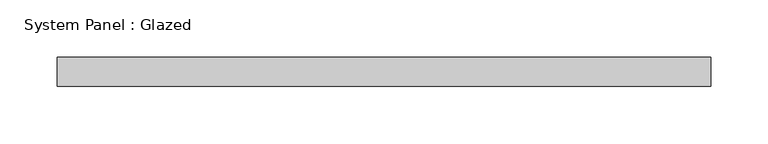
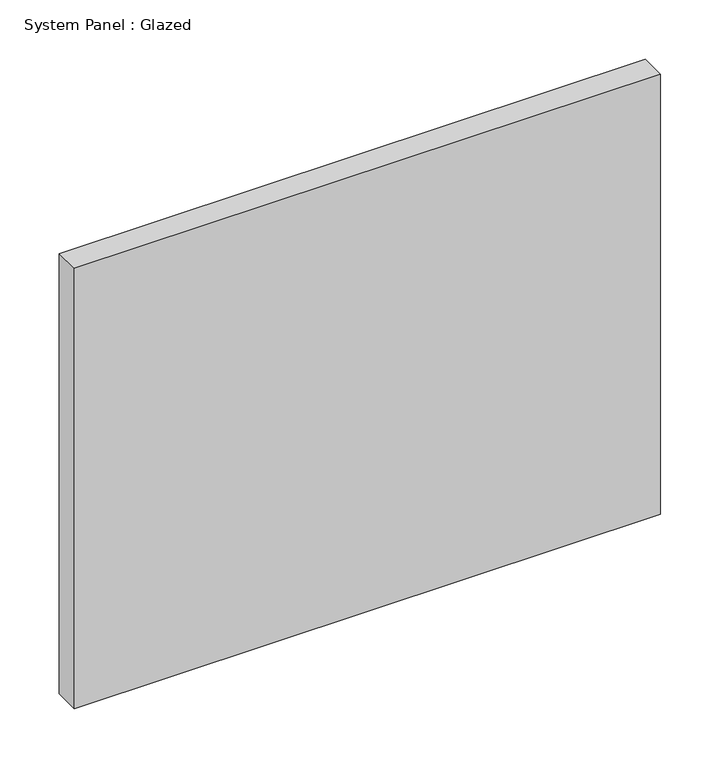
"""IFC4 building model written with IfcOpenShell, lengths in millimetres: plate geometry, System Panel : Glazed."""

from ifc_helpers import new_model, si_unit, origin, origin_with_axes, place, context, project, spatial, polyline, outline, extrude, source, transform, mapped, element, save


def system_panel_glazed_61a83ab7(model_context):
    return source(origin(), model_context, "Body", "SweptSolid", [
        extrude(outline(polyline([(285.75, 19.05), (-285.75, 19.05), (-285.75, 44.45), (285.75, 44.45), (285.75, 19.05)])), origin_with_axes(), (0.0, 0.0, 1.0), 453.5236842),
    ])


if __name__ == "__main__":
    model = new_model("IFC4")
    model_context = context("Model", 3, world=origin())
    ifc_project = project(units=[si_unit("LENGTHUNIT", "METRE", prefix="MILLI")], contexts=[model_context])
    site = spatial("IfcSite", under=ifc_project)
    building = spatial("IfcBuilding", under=site)
    placement = place(None, origin())
    system_panel_glazed_shape = system_panel_glazed_61a83ab7(model_context)
    element("IfcPlate", 1, ObjectType="System Panel : Glazed", at=placement, inside=building, context=model_context, shape_type="MappedRepresentation", body=[
        mapped(system_panel_glazed_shape, transform((0.0, 0.0, 0.0), x_axis=(1.0, 0.0, 0.0), y_axis=(0.0, 1.0, 0.0), z_axis=(0.0, 0.0, 1.0))),
    ])
    save(model, "model.ifc")

# Revit data of these elements
# Type "System Panel : Glazed"
#   Construction Type Id = "GSP4R"
#   Analytic Construction = "1/8 in Pilkington single glazing"
#   Visual Light Transmittance = 0.9
#   Solar Heat Gain Coefficient = 0.86
#   Heat Transfer Coefficient (U) = 1.18115 BTU/(h·ft²·°F)
#   Define Thermal Properties by = 1
# Element 1 (IfcPlate, "System Panel : Glazed")
#   Materials on its faces: "Glass"
# Materials
#   "Glass": class "Glass", colour RGB 0 128 192, transparency 0.75, Description = "Soda Lime Glass", Cost = 0
